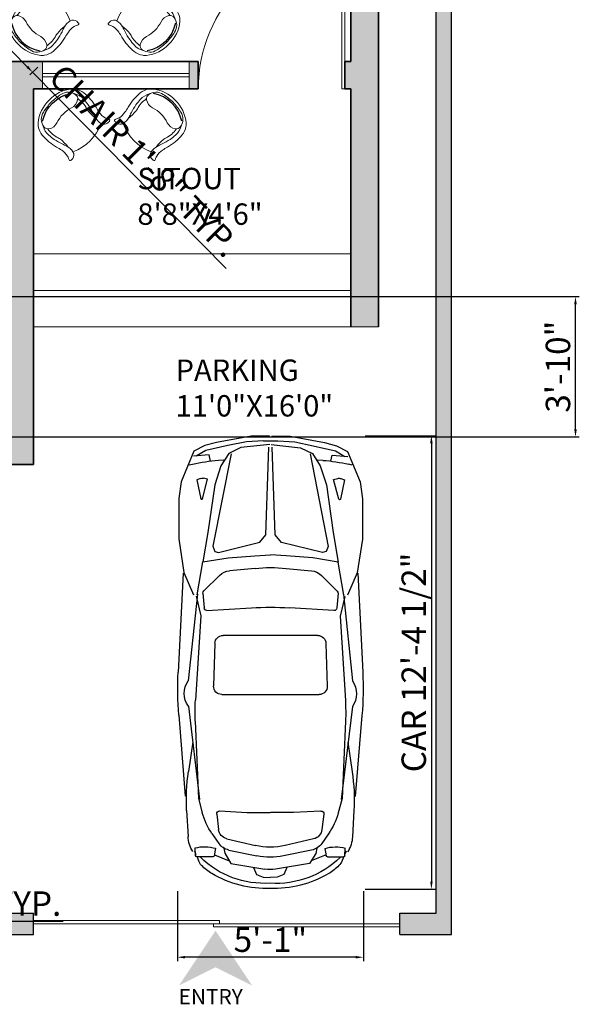
# Model space of a CAD drawing. Units: inches. Extents: x 2700 to 4052, y 1030 to 1872.
# Tile 2 of 8: x 3033 to 3217, y 1079 to 1401. Entities that reach past the tile are written whole.
import ezdxf

# ---------------------------------------------------------------- set-up
doc = ezdxf.new("R2010")
doc.units = ezdxf.units.IN
for name, color, linetype, lineweight in [('A-ANNO-DIMS', 2, 'Continuous', 13), ('A-ANNO-SYMB', 7, 'Continuous', 18), ('A-ANNO-TEXT', 7, 'Continuous', 18), ('A-AREA-IDEN', 7, 'Continuous', 18), ('A-DOOR', 4, 'Continuous', 18), ('A-FLOR-STRS', 7, 'Continuous', 18), ('A-FURN', 8, 'Continuous', 18), ('A-GLAZ', 4, 'Continuous', 18), ('A-WALL', 7, 'Continuous', 35), ('A-WALL-PATT', 7, 'Continuous', 13), ('C-PROP', 7, 'Continuous', 25), ('C-SITE-GATE', 7, 'Continuous', 18), ('C-SITE-VEHI', 8, 'Continuous', 13)]:
    doc.layers.add(name, color=color, linetype=linetype, lineweight=lineweight)
doc.layers.add('C-SITE-PATT', color=252, linetype='Continuous', lineweight=13, true_color=0x939598)
doc.layers.add('IFF-FURN-DETAIL', color=250, linetype='Continuous')
doc.layers.add('L9012X$0', color=2, linetype='Continuous')
doc.styles.get("Standard").update_dxf_attribs({"font": 'arial.ttf'})
doc.dimstyles.new('ISO-25', dxfattribs={"dimtxt": 8, "dimasz": 2.5, "dimexe": 1.25, "dimexo": 0.625, "dimtad": 1, "dimdec": 1, "dimlunit": 3, "dimtxsty": 'Standard', "dimcen": 2.5, "dimclrt": 1, "dimadec": 0, "dimazin": 0, "dimtfac": 1, "dimtdec": 1, "dimtmove": 0, "dimatfit": 3, "dimfxl": 1, "dimarcsym": 0})

# ---------------------------------------------------------------- blocks, each defined once
blk = doc.blocks.new('ILNG95')
for points in [[(120, 308, -0.32971), (51, 384, -0.036099), (50, 422, -0.497733), (75, 439, -0.070621), (96, 429, 0.101868), (133, 414, 0.091794), (259, 412, 0.024114), (351, 433, -0.090294), (638, 458, -0.132412), (775, 407, -0.068618), (816, 368, -0.184346), (943, 0, 1.803905)], [(120, 308, 0.138132), (244, 313, 0.001085), (325, 339, -0.034227), (462, 375, -0.033255), (567, 387, -0.137428), (727, 350, -4.561553)], [(120, 308, 0.138132), (244, 313, 0.001085), (325, 339, -0.034227), (462, 375, -0.033255), (567, 387, -0.137428), (727, 350, -4.561553)], [(235, 308, 0.064243), (394, 307, 0.04414), (433, 315, -0.118032), (643, 329, -6.296816)], [(235, 308, 0.064243), (394, 307, 0.04414), (433, 315, -0.118032), (643, 329, -6.296816)], [(639, 0, 0.078302), (612, 161, -0.233633), (633, 315, -0.28763), (710, 349, -0.317923), (875, 193, -0.032882), (900, 0, 1.140397)], [(639, 0, 0.078302), (612, 161, -0.233633), (633, 315, -0.28763), (710, 349, -0.317923), (875, 193, -0.032882), (900, 0, 1.140397)], [(120, -308, 0.32971), (51, -384, 0.036099), (50, -422, 0.497733), (75, -439, 0.070621), (96, -429, -0.101868), (133, -414, -0.091794), (259, -412, -0.024114), (351, -433, 0.090294), (638, -458, 0.132412), (775, -407, 0.068618), (816, -368, 0.184346), (943, 0, -1.803905)], [(639, 0, -0.078302), (612, -161, 0.233633), (633, -315, 0.28763), (710, -349, 0.317923), (875, -193, 0.032882), (900, 0, -1.140397)], [(639, 0, -0.078302), (612, -161, 0.233633), (633, -315, 0.28763), (710, -349, 0.317923), (875, -193, 0.032882), (900, 0, -1.140397)], [(120, -308, -0.138132), (244, -313, -0.001085), (325, -339, 0.034227), (462, -375, 0.033255), (567, -387, 0.137428), (727, -350, 4.561553)], [(120, -308, -0.138132), (244, -313, -0.001085), (325, -339, 0.034227), (462, -375, 0.033255), (567, -387, 0.137428), (727, -350, 4.561553)], [(235, -308, -0.064243), (394, -307, -0.04414), (433, -315, 0.118032), (643, -329, 6.296816)], [(235, -308, -0.064243), (394, -307, -0.04414), (433, -315, 0.118032), (643, -329, 6.296816)]]:
    blk.add_lwpolyline(points, format="xyb")
blk.add_arc((759, 1), 709, 154.3281, 205.801)
at = {"layer": 'IFF-FURN-DETAIL'}
blk.add_arc((326, -2), 549, 326.8997, 34.6691, dxfattribs=at)
blk.add_arc((326, -2), 549, 326.8997, 34.6691, dxfattribs=at)
blk = doc.blocks.new('A1099DC')
at = {"color": 0, "linetype": 'ByBlock'}
for p, q in [((1279.298465, 804.448389), (2201.430588, 851.890505)), ((2602.736326, 846.078152), (3356.693814, 785.353187)), ((272.228253, 749.073842), (265.114727, 718.465169)), ((1475.52921, 670.226262), (2282.402739, 758.004075)), ((2519.280414, 756.817792), (3387.476361, 653.818028)), ((2851.341839, 715.213377), (3126.60716, 755.701993)), ((3488.458929, 772.663345), (3732.658862, 759.86454)), ((139.051458, 595.027331), (190.951238, 683.213377)), ((179.200345, 564.515703), (190.951238, 709.631982)), ((398.733388, 644.315148), (411.280494, 678.748261)), ((411.280494, 678.748261), (588.616917, 641.417897)), ((1482.852352, 674.283145), (1175.286956, 622.180789)), ((1494.603245, 682.841284), (1678.210958, 641.166865)), ((1678.210958, 641.166865), (2462.684993, 690.847736)), ((2656.476214, 692.831247), (3376.704709, 662.004075)), ((3376.704709, 662.004075), (3510.708679, 626.736433)), ((3909.27561, 688.812956), (3837.725727, 693.401722)), ((3867.794139, 700.329656), (3900.059395, 686.767505)), ((3921.162781, 527.618662), (3921.162781, 676.138994)), ((3925.383812, 676.122818), (3955.306409, 663.545364)), ((92.537504, 388.14361), (139.051458, 595.027331)), ((236.043912, 551.980927), (179.200345, 564.515703)), ((405.405047, 577.538958), (396.874865, 615.894428)), ((589.014326, 626.599587), (405.405047, 577.538958)), ((1300.814287, 466.658131), (1445.712032, 613.104998)), ((1465.665584, 620.56924), (1602.893878, 610.287296)), ((1626.354615, 583.507504), (1602.652901, 169.222264)), ((229.117398, 477.634662), (225.714299, 427.957563)), ((1933.148906, 509.557888), (2330.980062, 522.200075)), ((3493.960271, 465.734554), (3507.923021, 209.166865)), ((3522.252709, 492.345257), (3666.066199, 475.644444)), ((3704.596898, 536.993674), (3795.675135, 473.385795)), ((3841.786866, 503.451367), (3910.58243, 515.096797)), ((3901.001848, 514.780764), (3957.150905, 375.772812)), ((57.774444, 216.608726), (92.537504, 388.14361)), ((1235.045743, 136.116317), (1257.419842, 373.755108)), ((1860.238743, -448.635916), (1859.369151, 433.397797)), ((2409.60024, 445.938054), (2410.49349, -460.09121)), ((3753.293176, 397.789551), (3815.226005, 132.124765)), ((3839.396146, 426.841284), (3888.358202, 417.538958)), ((3857.610793, 379.525702), (3912.067615, 118.157673)), ((3888.358202, 417.538958), (3983.199613, 359.957848)), ((3983.199613, 359.957848), (4035.448301, 43.94997)), ((49.168662, 58.00681), (57.774444, 216.608726)), ((3507.923021, 209.166865), (3507.64153, -4.333678)), ((4019.086894, 150.376168), (4084.69605, 122.469191)), ((4084.69605, 122.469191), (4109.177079, 60.329656)), ((4109.177079, 60.329656), (4113.094043, -5.158716)), ((49.301278, -76.507426), (58.219773, -235.092064)), ((3508.347273, -221.154823), (3507.644805, -7.65525)), ((3983.920268, -371.008369), (4035.545755, -54.898082)), ((4084.948231, -133.320044), (4109.306686, -71.132359)), ((4109.306686, -71.132359), (4113.094514, -5.636391)), ((1235.330373, -152.586046), (1258.173002, -390.180259)), ((3754.088875, -409.293325), (3815.497749, -143.506937)), ((3858.370276, -390.823819), (3912.311631, -129.348921)), ((4019.394229, -161.356334), (4084.948231, -133.320044)), ((58.219773, -235.092064), (93.320996, -406.558069)), ((1627.520644, -599.204785), (1603.002095, -184.967086)), ((3494.890446, -477.749545), (3508.347273, -221.154823)), ((93.320996, -406.558069), (140.24279, -613.349673)), ((230.077082, -495.779641), (226.576036, -446.109349)), ((3840.248961, -438.175225), (3889.19258, -428.776374)), ((3889.19258, -428.776374), (3983.920268, -371.008369)), ((3902.027941, -525.993061), (3957.902795, -386.874665)), ((1301.750547, -482.997536), (1446.936772, -629.158411)), ((1934.168526, -524.650381), (2332.023837, -536.508105)), ((3523.2353, -504.304409), (3667.01558, -487.320059)), ((3705.667171, -548.593196), (3796.61981, -484.805853)), ((3842.790735, -514.780444), (3911.609128, -526.290202)), ((3922.214148, -538.79118), (3922.506998, -687.311224)), ((140.24279, -613.349673), (192.316354, -701.433212)), ((237.150178, -570.112104), (180.331436, -582.758939)), ((180.331436, -582.758939), (192.368445, -727.851766)), ((406.561378, -595.336142), (398.106841, -633.708356)), ((590.267037, -644.034637), (406.561378, -595.336142)), ((1484.19765, -690.263206), (1176.530118, -638.767405)), ((1466.905004, -636.583294), (1604.112757, -626.030785)), ((3378.022114, -674.249887), (3511.956283, -638.718087)), ((400.0214, -662.125356), (412.636377, -696.533662)), ((412.636377, -696.533662), (589.898847, -658.853701)), ((1476.866524, -686.22077), (2283.911563, -772.40743)), ((1495.965396, -698.798158), (1679.490579, -656.761786)), ((1679.490579, -656.761786), (2464.061049, -704.895745)), ((2520.786439, -770.754078), (3388.777604, -666.042617)), ((2657.855804, -706.497136), (3378.022114, -674.249887)), ((2852.765183, -728.494989), (3128.109803, -768.440762)), ((3910.644841, -700.0086), (3839.104145, -704.738438)), ((3869.186159, -711.60707), (3901.424611, -697.981326)), ((3926.727989, -687.286725), (3956.625729, -674.650294)), ((273.723073, -767.133288), (266.549207, -736.538701)), ((1280.900818, -820.829563), (2203.124693, -866.453338)), ((2604.418191, -859.849707), (3358.254477, -797.638217)), ((3489.994314, -784.688586), (3734.168535, -771.408296))]:
    blk.add_line(p, q, dxfattribs=at)
for points in [[(-0.000783, 0.794772), (5.385043, 172.701749), (63.649891, 493.818028), (92.537504, 603.957563), (144.437284, 705.166865), (428.417214, 824.236633), (585.095796, 846.190121), (961.406447, 846.190121), (1274.27399, 797.818028), (1482.852352, 709.631982)], [(83.345007, -3.206171), (111.32237, 268.957533), (164.563706, 379.583828), (279.999271, 453.709838), (456.549665, 511.628518), (901.254996, 574.918954), (1175.286956, 622.180789), (1137.52997, 385.548359), (1118.345181, 137.317882), (1109.829198, -8.358455)], [(168.178729, 359.003083), (1030.214866, 528.397865), (1077.798844, 510.531569), (1086.170082, 475.285426), (992.832238, 91.960378), (924.218938, 35.478085), (108.447994, 6.034416)], [(0.019119, -19.392451), (5.743899, -191.288474), (64.641806, -512.289243), (93.746535, -622.371603), (145.845778, -723.478374), (430.059935, -841.987962), (586.7815, -863.632471), (963.091723, -863.198028), (1275.863278, -814.209121), (1484.26735, -725.611974)], [(83.356858, -15.227176), (111.870816, -287.335185), (165.330179, -397.856284), (280.911681, -471.754535), (457.575935, -529.324983), (902.4055, -592.045995), (1176.530118, -638.767405), (1138.306616, -402.209884), (1118.632407, -154.017717), (1109.829198, -8.358455)], [(168.904615, -377.268451), (1031.273389, -545.270714), (1078.822046, -527.310627), (1087.123771, -492.048047), (993.030273, -108.907787), (924.305735, -52.560894), (108.478017, -24.418246)]]:
    blk.add_lwpolyline(points, dxfattribs=at)
for centre, radius, start, end in [((2358.037832, -2192.08357), 3048, 85.395244, 92.945173), ((2399.99649, 588.663508), 206.166238, 54.649181, 124.776949), ((3392.740754, -1053.630025), 1828.8, 86.999806, 98.367602), ((3718.678317, 475.802507), 284.405862, 57.329946, 87.182375), ((1749.553982, 373.478072), 1524, 166.916578, 176.08111), ((446.46332, 626.922805), 50.8, 159.97873, 192.538409), ((2578.271641, -1134.295865), 1828.8, 87.549126, 93.623712), ((4191.049821, 605.937201), 363.988953, 166.096081, 196.353514), ((3908.462781, 676.138994), 12.7, 0, 86.330429), ((3320.85101, 50.338397), 847.430844, 356.245089, 44.519453), ((3896.252417, 523.051998), 152.4, 46.38363, 67.20138), ((587.047263, 633.961317), 7.62, 284.960009, 78.112462), ((1463.767788, 595.240237), 25.4, 85.715073, 135.304647), ((1600.996082, 584.958293), 25.4, 356.725615, 85.715073), ((3355.555414, 37.211519), 609.6, 55.070043, 75.255062), ((3700.933354, 318.064082), 435.542335, 30.457681, 46.38363), ((1409.148822, 359.469565), 152.4, 135.304647, 174.62136), ((1935.569151, 433.396333), 76.2, 91.82012, 179.9989), ((2333.400307, 446.03852), 76.2, 359.924458, 91.82012), ((3519.322741, 467.114813), 25.4, 83.37601, 183.115039), ((3654.346327, 374.722669), 101.6, 13.122645, 83.37601), ((3708.414764, 348.440256), 152.4, 11.769371, 55.070043), ((3908.462781, 527.618662), 12.7, 279.607718, 0), ((3204.184594, 25.950693), 1011.814461, 358.069446, 30.457681), ((2752.335538, -6.739118), 1524, 174.62136, 185.491615), ((4645.676894, -4.872483), 3048, 176.725615, 183.38736), ((3221.54491, -6.276527), 609.6, 346.99033, 13.122645), ((3315.283499, -6.18411), 609.6, 348.343604, 11.769371), ((1266.577845, -8.050136), 1219.2, 176.894161, 183.218814), ((3734.73098, -5.770579), 304.8, 350.724636, 9.388339), ((3320.962449, -62.69553), 847.430844, 315.593523, 3.867886), ((3204.248172, -38.537915), 1011.814461, 329.655294, 2.043529), ((1409.873518, -375.595566), 152.4, 185.491615, 224.808328), ((1936.438592, -448.484202), 76.2, 180.114076, 268.292856), ((3655.096735, -386.42159), 101.6, 276.736965, 346.99033), ((3709.113243, -360.032616), 152.4, 305.042932, 348.343604), ((1750.305335, -388.625277), 1524, 184.031865, 193.196397), ((2334.293902, -460.341926), 76.2, 268.292856, 0.188517), ((3520.255588, -479.079792), 25.4, 176.997936, 276.736965), ((3355.640902, -49.500248), 609.6, 284.857913, 305.042932), ((4192.255091, -616.577407), 363.988953, 163.759461, 194.016894), ((3909.514173, -538.816222), 12.7, 0.112975, 80.505257), ((3701.571953, -329.671253), 435.542335, 313.729345, 329.655294), ((447.716945, -644.638934), 50.8, 167.574566, 200.134245), ((1464.957267, -611.258083), 25.4, 224.808328, 274.397903), ((1602.165021, -600.705574), 25.4, 274.397903, 3.38736), ((588.314493, -651.400231), 7.62, 282.000513, 75.152966), ((2576.048678, 1120.472221), 1828.8, 266.489263, 272.563849), ((3719.627907, -487.374382), 284.405862, 272.930601, 302.78303), ((3909.807023, -687.336265), 12.7, 273.782546, 0.112975), ((3897.294828, -534.273643), 152.4, 292.911596, 313.729345), ((2401.171182, -602.835323), 206.166238, 235.336026, 305.463794), ((3390.675263, 1041.412497), 1828.8, 261.745373, 273.113169), ((2353.729565, 2177.823616), 3048, 267.167802, 274.717731)]:
    blk.add_arc(centre, radius, start, end, dxfattribs=at)
blk = doc.blocks.new('VI')
at = {"layer": 'L9012X$0'}
blk.add_blockref('A1099DC', (0, 0), dxfattribs=at)
blk = doc.blocks.new('DOOR-SWING-48IN')
for p, q in [((-1, 48), (-1, 0)), ((0, 48), (0, 0)), ((0, 0), (-1, 0))]:
    blk.add_line(p, q)
blk.add_arc((0, 0), 48, 90, 180)
blk = doc.blocks.new('WINDOW-48IN')
for p, q in [((-24, -4.5), (-24, 4.5)), ((24, -4.5), (24, 4.5)), ((-24, 0.5), (24, 0.5)), ((-24, -0.5), (24, -0.5))]:
    blk.add_line(p, q)
blk = doc.blocks.new('GATE-SLIDING-120IN')
for p, q in [((0, 2), (61, 2)), ((0, 1), (120, 1)), ((59, 1), (59, 0)), ((59, 0), (120, 0)), ((61, 2), (61, 1))]:
    blk.add_line(p, q)
blk = doc.blocks.new('*D82')
at = {"layer": 'A-ANNO-DIMS', "color": 0, "lineweight": -2, "transparency": 16777216}
for p, q in [((3025.17, 1399.72), (3022.61, 1397.19)), ((3025.25, 1396.29), (3035.65, 1385.75)), ((3039.07, 1385.62), (3036.51, 1383.09)), ((3037.4, 1383.97), (3100.81, 1319.68))]:
    blk.add_line(p, q, dxfattribs=at)
at = {"layer": 'A-ANNO-DIMS', "color": 0, "transparency": 16777216}
for points in [[(3025.55, 1396.58), (3024.96, 1396), (3023.5, 1398.07)], [(3035.95, 1386.04), (3035.35, 1385.46), (3037.4, 1383.97)]]:
    blk.add_solid(points, dxfattribs=at)
at = {"layer": 'Defpoints', "color": 0, "transparency": 16777216}
for p in [(3025.61, 1400.16), (3037.4, 1383.97), (3039.52, 1386.06)]:
    blk.add_point(p, dxfattribs=at)
at = {"layer": 'A-ANNO-DIMS', "color": 1, "transparency": 16777216, "insert": (3073.38, 1354.28), "char_height": 8, "attachment_point": 5, "rotation": 314.6051}
blk.add_mtext('CHAIR 1\'-8" TYP.', dxfattribs=at)
blk = doc.blocks.new('*D83')
at = {"layer": 'A-ANNO-DIMS', "color": 0, "lineweight": -2, "transparency": 16777216}
for p, q in [((3039.09, 1414.33), (3036.56, 1416.89)), ((3035.66, 1414.24), (3025.31, 1404.03)), ((3023.53, 1402.27), (2973.4, 1352.84)), ((3025.17, 1400.6), (3022.65, 1403.16))]:
    blk.add_line(p, q, dxfattribs=at)
at = {"layer": 'A-ANNO-DIMS', "color": 0, "transparency": 16777216}
for points in [[(3035.37, 1414.54), (3035.95, 1413.94), (3037.44, 1416)], [(3025.01, 1404.33), (3025.6, 1403.73), (3023.53, 1402.27)]]:
    blk.add_solid(points, dxfattribs=at)
at = {"layer": 'Defpoints', "color": 0, "transparency": 16777216}
for p in [(3039.52, 1413.88), (3023.53, 1402.27), (3025.61, 1400.16)]:
    blk.add_point(p, dxfattribs=at)
at = {"layer": 'A-ANNO-DIMS', "color": 1, "transparency": 16777216, "insert": (2994.23, 1380.07), "char_height": 8, "attachment_point": 5, "rotation": 44.6051}
blk.add_mtext('1\'-7 1/2" TYP.', dxfattribs=at)
blk = doc.blocks.new('*D89')
at = {"layer": 'A-ANNO-DIMS', "color": 0, "lineweight": -2, "transparency": 16777216}
for p, q in [((2922.49, 1112.32), (2922.49, 1104.55)), ((2969.98, 1112.32), (2969.98, 1104.55)), ((2924.99, 1105.8), (2967.48, 1105.8)), ((2969.98, 1105.8), (3047.35, 1105.8))]:
    blk.add_line(p, q, dxfattribs=at)
at = {"layer": 'A-ANNO-DIMS', "color": 0, "transparency": 16777216}
for points in [[(2924.99, 1106.22), (2924.99, 1105.38), (2922.49, 1105.8)], [(2967.48, 1106.22), (2967.48, 1105.38), (2969.98, 1105.8)]]:
    blk.add_solid(points, dxfattribs=at)
at = {"layer": 'Defpoints', "color": 0, "transparency": 16777216}
for p in [(2922.49, 1112.94), (2969.98, 1112.94), (2969.98, 1105.8)]:
    blk.add_point(p, dxfattribs=at)
at = {"layer": 'A-ANNO-DIMS', "color": 1, "transparency": 16777216, "insert": (3009.92, 1110.57), "char_height": 8, "attachment_point": 5}
blk.add_mtext('3\'-11 1/2" TYP.', dxfattribs=at)
blk = doc.blocks.new('*D102')
at = {"layer": 'A-ANNO-DIMS', "color": 0, "lineweight": -2, "transparency": 16777216}
for p, q in [((3146.39, 1264.91), (3169.31, 1264.91)), ((3168.06, 1262.41), (3168.06, 1118.83)), ((3146.39, 1116.33), (3169.31, 1116.33))]:
    blk.add_line(p, q, dxfattribs=at)
at = {"layer": 'A-ANNO-DIMS', "color": 0, "transparency": 16777216}
for points in [[(3167.64, 1262.41), (3168.47, 1262.41), (3168.06, 1264.91)], [(3167.64, 1118.83), (3168.47, 1118.83), (3168.06, 1116.33)]]:
    blk.add_solid(points, dxfattribs=at)
at = {"layer": 'Defpoints', "color": 0, "transparency": 16777216}
for p in [(3145.77, 1264.91), (3145.77, 1116.33), (3168.06, 1116.33)]:
    blk.add_point(p, dxfattribs=at)
at = {"layer": 'A-ANNO-DIMS', "color": 1, "transparency": 16777216, "insert": (3163.3, 1190.62), "char_height": 8, "attachment_point": 5, "rotation": 90}
blk.add_mtext('CAR 12\'-4 1/2"', dxfattribs=at)
blk = doc.blocks.new('*D103')
at = {"layer": 'A-ANNO-DIMS', "color": 0, "lineweight": -2, "transparency": 16777216}
for p, q in [((3084.83, 1115.7), (3084.83, 1092.79)), ((3145.77, 1115.7), (3145.77, 1092.79)), ((3143.27, 1094.04), (3087.33, 1094.04))]:
    blk.add_line(p, q, dxfattribs=at)
at = {"layer": 'A-ANNO-DIMS', "color": 0, "transparency": 16777216}
for points in [[(3087.33, 1094.46), (3087.33, 1093.63), (3084.83, 1094.04)], [(3143.27, 1094.46), (3143.27, 1093.63), (3145.77, 1094.04)]]:
    blk.add_solid(points, dxfattribs=at)
at = {"layer": 'Defpoints', "color": 0, "transparency": 16777216}
for p in [(3084.83, 1116.33), (3145.77, 1116.33), (3084.83, 1094.04)]:
    blk.add_point(p, dxfattribs=at)
at = {"layer": 'A-ANNO-DIMS', "color": 1, "transparency": 16777216, "insert": (3115.3, 1098.75), "char_height": 8, "attachment_point": 5}
blk.add_mtext('5\'-1"', dxfattribs=at)
blk = doc.blocks.new('*D114')
at = {"layer": 'A-ANNO-DIMS', "color": 0, "lineweight": -2, "transparency": 16777216}
for p, q in [((2872.29, 1310.49), (3216.52, 1310.49)), ((3215.27, 1267.02), (3215.27, 1307.99)), ((2872.29, 1264.52), (3216.52, 1264.52))]:
    blk.add_line(p, q, dxfattribs=at)
at = {"layer": 'A-ANNO-DIMS', "color": 0, "transparency": 16777216}
for points in [[(3214.85, 1307.99), (3215.69, 1307.99), (3215.27, 1310.49)], [(3214.85, 1267.02), (3215.69, 1267.02), (3215.27, 1264.52)]]:
    blk.add_solid(points, dxfattribs=at)
at = {"layer": 'Defpoints', "color": 0, "transparency": 16777216}
for p in [(2871.67, 1310.49), (3215.27, 1310.49), (2871.67, 1264.52)]:
    blk.add_point(p, dxfattribs=at)
at = {"layer": 'A-ANNO-DIMS', "color": 1, "transparency": 16777216, "insert": (3210.56, 1287.51), "char_height": 8, "attachment_point": 5, "rotation": 90}
blk.add_mtext('3\'-10"', dxfattribs=at)

msp = doc.modelspace()

# ---------------------------------------------------------------- hatches: boundary and pattern name
at = {"layer": 'A-ANNO-SYMB'}
h = msp.add_hatch(color=256, dxfattribs=at)
h.dxf.hatch_style = 1
h.paths.add_polyline_path([(3097.33, 1090.74), (3109.33, 1084.74), (3097.33, 1102.74), (3085.33, 1084.74)])
at = {"layer": 'A-WALL-PATT'}
h = msp.add_hatch(color=256, dxfattribs=at)
h.dxf.hatch_style = 1
h.paths.add_polyline_path([(2814.67, 1264.52), (2814.67, 1168.52), (2955.67, 1168.52), (2955.67, 1177.52), (2823.67, 1177.52), (2823.67, 1255.52), (2897.67, 1255.52), (2897.67, 1264.52), (2871.67, 1264.52), (2871.67, 1310.49), (2862.67, 1310.49), (2862.67, 1304.37), (2862.67, 1264.52)])
h.paths.add_polyline_path([(2945.67, 1255.52), (2986.67, 1255.52), (2986.67, 1264.52), (2980.67, 1264.52), (2980.67, 1324.52), (3028.67, 1324.52), (3028.67, 1264.52), (3022.67, 1264.52), (3022.67, 1255.52), (3037.67, 1255.52), (3037.67, 1378.52), (3040.67, 1378.52), (3040.67, 1387.52), (3022.67, 1387.52), (3022.67, 1381.52), (3028.67, 1381.52), (3028.67, 1333.52), (2980.67, 1333.52), (2980.67, 1381.52), (2986.67, 1381.52), (2986.67, 1387.52), (2971.67, 1387.52), (2971.67, 1264.52), (2945.67, 1264.52)])
h.paths.add_polyline_path([(2871.67, 1358.49), (2871.67, 1382.52), (2862.67, 1382.52), (2862.67, 1358.49)])
h.paths.add_polyline_path([(3091.67, 1387.52), (3088.67, 1387.52), (3088.67, 1378.52), (3091.67, 1378.52)])
h.paths.add_polyline_path([(3141.67, 1300.52), (3150.67, 1300.52), (3150.67, 1431.52), (3141.67, 1431.52), (3141.67, 1387.52), (3139.67, 1387.52), (3139.67, 1378.52), (3141.67, 1378.52)])
h.paths.add_polyline_path([(2830.28, 1565.14), (2830.28, 1604.05), (2822.03, 1604.05), (2822.03, 1565.14)], flags=9)
h.paths.add_polyline_path([(2957.35, 1565.68), (2957.35, 1611.46), (2949.11, 1611.46), (2949.11, 1565.68)], flags=9)
h.paths.add_polyline_path([(2983.54, 1697.89), (2983.54, 1743.66), (2975.29, 1743.66), (2975.29, 1697.89)], flags=9)
h.paths.add_polyline_path([(2879.08, 1800.61), (2924.85, 1800.61), (2924.85, 1808.85), (2879.08, 1808.85)], flags=9)
h.paths.add_polyline_path([(2815.49, 1361.72), (2864.45, 1361.72), (2864.45, 1388.34), (2815.49, 1388.34)], flags=9)
h.paths.add_polyline_path([(2904.6, 1318.27), (2953.91, 1318.27), (2953.91, 1344.89), (2904.6, 1344.89)], flags=9)
h.paths.add_polyline_path([(3036.9, 1507.34), (3091.04, 1507.34), (3091.04, 1533.96), (3036.9, 1533.96)], flags=9)
h.paths.add_polyline_path([(2990.4, 1774.23), (3040.41, 1774.23), (3040.41, 1800.84), (2990.4, 1800.84)], flags=9)
h.paths.add_polyline_path([(3076.88, 1774.23), (3126.96, 1774.23), (3126.96, 1800.84), (3076.88, 1800.84)], flags=9)
h.paths.add_polyline_path([(3036.9, 1664.37), (3100.88, 1664.37), (3100.88, 1690.98), (3036.9, 1690.98)], flags=9)
h.paths.add_polyline_path([(2871.85, 1747.79), (2935.82, 1747.79), (2935.82, 1774.41), (2871.85, 1774.41)], flags=9)
h.paths.add_polyline_path([(2871.85, 1590.97), (2935.82, 1590.97), (2935.82, 1617.58), (2871.85, 1617.58)], flags=9)
h.paths.add_polyline_path([(2862.5, 1447.4), (2911.46, 1447.4), (2911.46, 1474.01), (2862.5, 1474.01)], flags=9)
at = {"layer": 'C-SITE-PATT'}
h = msp.add_hatch(color=256, dxfattribs=at)
h.dxf.hatch_style = 1
h.paths.add_polyline_path([(2819.67, 1821.52), (2814.67, 1821.52), (2814.67, 1423.52), (2819.67, 1423.52)])
h.paths.add_polyline_path([(3037.67, 1108.52), (2819.67, 1108.52), (2819.67, 1168.52), (2814.67, 1168.52), (2814.67, 1101.52), (3037.67, 1101.52)])
h.paths.add_polyline_path([(3174.67, 1821.52), (3169.67, 1821.52), (3169.67, 1108.52), (3157.67, 1108.52), (3157.67, 1101.52), (3174.67, 1101.52)])

# ---------------------------------------------------------------- linework, layer by layer
at = {"layer": 'A-FLOR-STRS'}
for p, q in [((3141.67, 1324.52), (3037.67, 1324.52)), ((3141.67, 1312.52), (3037.67, 1312.52)), ((3150.67, 1300.52), (3037.67, 1300.52))]:
    msp.add_line(p, q, dxfattribs=at)
at = {"layer": 'A-WALL'}
for p, q in [((3150.67, 1300.52), (3150.67, 1821.52)), ((3141.67, 1387.52), (3141.67, 1627.52)), ((3091.67, 1387.52), (3022.67, 1387.52)), ((3091.67, 1378.52), (3091.67, 1387.52)), ((3141.67, 1387.52), (3139.67, 1387.52)), ((3139.67, 1378.52), (3139.67, 1387.52)), ((3037.67, 1255.52), (3037.67, 1378.52)), ((3091.67, 1378.52), (3037.67, 1378.52)), ((3141.67, 1378.52), (3139.67, 1378.52)), ((3141.67, 1300.52), (3141.67, 1378.52)), ((3037.67, 1255.52), (3022.67, 1255.52))]:
    msp.add_line(p, q, dxfattribs=at)
at = {"layer": 'C-PROP'}
for p, q in [((3169.67, 1108.52), (3169.67, 1821.52)), ((2819.67, 1108.52), (3037.67, 1108.52)), ((3037.67, 1101.52), (3037.67, 1108.52)), ((3157.67, 1101.52), (3157.67, 1108.52)), ((3157.67, 1108.52), (3169.67, 1108.52))]:
    msp.add_line(p, q, dxfattribs=at)
msp.add_lwpolyline([(3157.67, 1101.52), (3174.67, 1101.52), (3174.67, 1821.52), (2814.67, 1821.52), (2814.67, 1101.52), (3037.67, 1101.52)], dxfattribs=at)

# ---------------------------------------------------------------- block references
at = {"layer": 'A-DOOR'}
msp.add_blockref('DOOR-SWING-48IN', (3139.67, 1378.52), dxfattribs=at)
at = {"layer": 'A-FURN', "yscale": 0.0212192471586889, "zscale": 0.0212192471586889}
for p, xscale, rotation in [((3046.88, 1407.22), 0.0212192471586889, 224.6051083961163), ((3067.81, 1407.22), -0.0212192471586889, 135.3948916038836), ((3057.01, 1360.77), -0.0212192471586889, 315.3948916038837), ((3069.86, 1360.77), 0.0212192471586889, 44.60510839611638)]:
    msp.add_blockref('ILNG95', p, dxfattribs=dict(at, xscale=xscale, rotation=rotation))
at = {"layer": 'A-GLAZ'}
msp.add_blockref('WINDOW-48IN', (3064.67, 1383.02), dxfattribs=at)
at = {"layer": 'C-SITE-GATE'}
msp.add_blockref('GATE-SLIDING-120IN', (3037.67, 1104.02), dxfattribs=at)
at = {"layer": 'C-SITE-VEHI', "xscale": -0.0351896714874634, "yscale": 0.0351896714874634, "zscale": 0.0351896714874634, "rotation": 90}
msp.add_blockref('VI', (3115.05, 1264.91), dxfattribs=at)

# ---------------------------------------------------------------- texts
at = {"layer": 'A-ANNO-TEXT', "insert": (3085.25, 1083.62), "char_height": 5, "attachment_point": 1}
msp.add_mtext_dynamic_manual_height_columns('{\\fTimes New Roman|b0|i0|c0|p18;ENTRY}', width=196.2607, gutter_width=12.5, heights=[0], dxfattribs=at)
at = {"layer": 'A-AREA-IDEN', "char_height": 7, "attachment_point": 1}
for s, insert in [('{\\fTimes New Roman|b0|i0|c0|p18;SITOUT\\P8\'8"X4\'6"}', (3071.71, 1352.66)), ('{\\fTimes New Roman|b0|i0|c0|p18;PARKING\\P11\'0"X16\'0"}', (3084.23, 1289.86))]:
    msp.add_mtext_dynamic_manual_height_columns(s, width=61.0557, gutter_width=12.5, heights=[0], dxfattribs=dict(at, insert=insert))

# ---------------------------------------------------------------- dimensions: what is measured, and where the dimension line sits
at = {"layer": 'A-ANNO-DIMS'}
for base, p1, p2, angle, text, picture, middle in [((3023.53, 1402.27), (3039.52, 1413.88), (3025.61, 1400.16), 224.6051, '<> TYP.', '*D83', (2994.23, 1380.07)), ((3037.4, 1383.97), (3025.61, 1400.16), (3039.52, 1386.06), 314.6051, 'CHAIR <> TYP.', '*D82', (3073.38, 1354.28)), ((3168.06, 1116.33), (3145.77, 1264.91), (3145.77, 1116.33), 270, 'CAR <>', '*D102', (3163.3, 1190.62))]:
    dim = msp.add_linear_dim(base=base, p1=p1, p2=p2, angle=angle, text=text, dimstyle='ISO-25', override={"dimdec": 1, "dimlfac": 1, "dimrnd": 0, "dimzin": 1, "dimdsep": 46, "dimlunit": 4, "dimfrac": 2}, dxfattribs=at)
    dim.commit()
    dim.dimension.update_dxf_attribs({"geometry": picture, "text_midpoint": middle})
for base, p1, p2, angle, picture, middle in [((3215.27, 1310.49), (2871.67, 1264.52), (2871.67, 1310.49), 90, '*D114', (3210.56, 1287.51)), ((3084.83, 1094.04), (3145.77, 1116.33), (3084.83, 1116.33), 180, '*D103', (3115.3, 1098.75))]:
    dim = msp.add_linear_dim(base=base, p1=p1, p2=p2, angle=angle, dimstyle='ISO-25', override={"dimdec": 1, "dimlfac": 1, "dimrnd": 0, "dimzin": 1, "dimdsep": 46, "dimlunit": 4, "dimfrac": 2}, dxfattribs=at)
    dim.commit()
    dim.dimension.update_dxf_attribs({"geometry": picture, "text_midpoint": middle})
dim = msp.add_linear_dim(base=(2969.98, 1105.8), p1=(2922.49, 1112.94), p2=(2969.98, 1112.94), text='<> TYP.', dimstyle='ISO-25', override={"dimdec": 1, "dimlfac": 1, "dimrnd": 0, "dimzin": 1, "dimdsep": 46, "dimlunit": 4, "dimfrac": 2}, dxfattribs=at)
dim.commit()
dim.dimension.update_dxf_attribs({"geometry": '*D89', "text_midpoint": (3009.92, 1110.57)})

doc.saveas('drawing.dxf')
